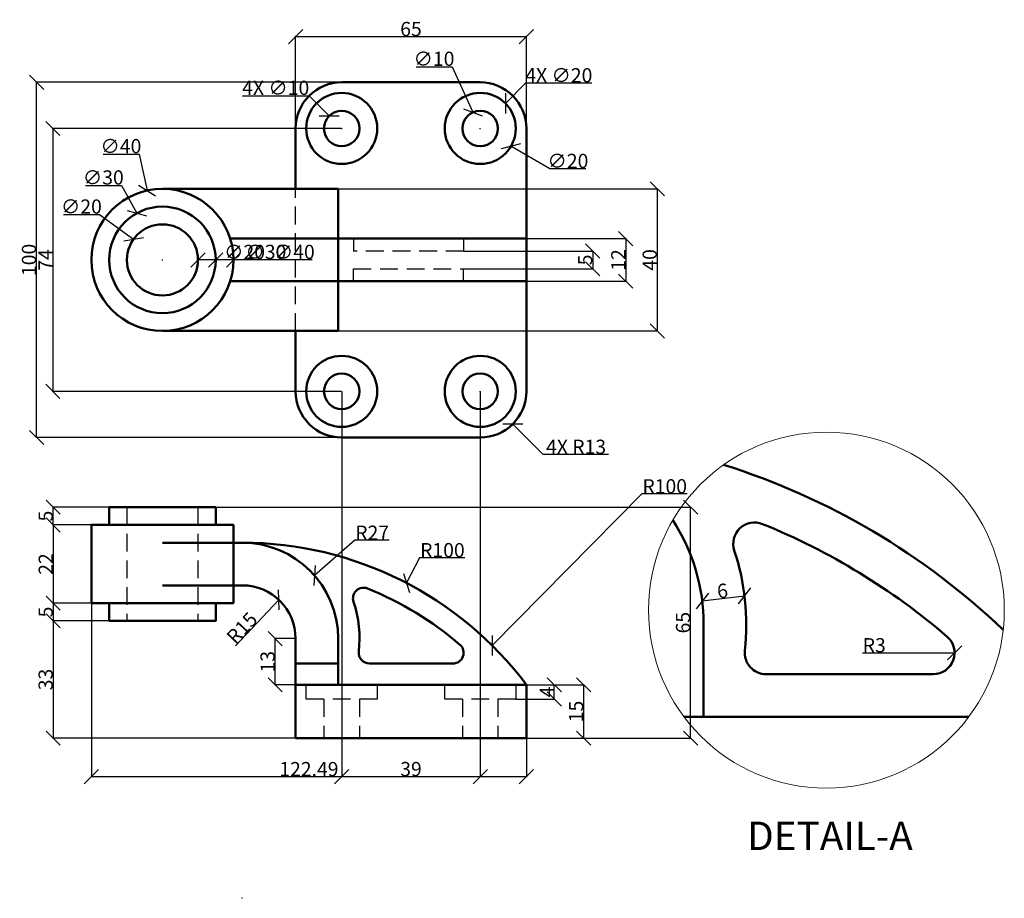
# Model space of a CAD drawing. Units: millimetres. Extents: x 103 to 380, y 45 to 292.
import ezdxf

# ---------------------------------------------------------------- set-up
doc = ezdxf.new("R2010")
doc.units = ezdxf.units.MM
doc.header["$MEASUREMENT"] = 0
doc.linetypes.add('HIDDEN', pattern=[0.375, 0.25, -0.125])
for name, color, linetype, lineweight in [('M-ANNO-DETL', 7, 'Continuous', 18), ('M-DIMS', 2, 'Continuous', 25), ('M-HIDN', 8, 'HIDDEN', 25), ('M-OUTL', 7, 'Continuous', 50), ('M-TEXT', 7, 'Continuous', 25)]:
    doc.layers.add(name, color=color, linetype=linetype, lineweight=lineweight)
doc.styles.get("Standard").update_dxf_attribs({"font": 'arial.ttf'})
doc.dimstyles.get("Standard").update_dxf_attribs({"dimtxt": 4, "dimasz": 4, "dimexe": 0.18, "dimexo": 0.0625, "dimgap": 0.09, "dimtad": 1, "dimtoh": 1, "dimdec": 0, "dimzin": 0, "dimdsep": 46, "dimtxsty": 'Standard', "dimblk": 'OBLIQUE', "dimcen": 0.09, "dimclre": 251, "dimadec": 0, "dimazin": 0, "dimtfac": 1, "dimtdec": 0, "dimtofl": 0, "dimtmove": 0, "dimatfit": 3, "dimfxl": 1, "dimtolj": 1, "dimtzin": 0, "dimarcsym": 0})

# ---------------------------------------------------------------- blocks, each defined once
blk = doc.blocks.new('_Oblique')
at = {"color": 0, "linetype": 'ByBlock', "lineweight": -2}
blk.add_line((-0.5, -0.5), (0.5, 0.5), dxfattribs=at)
blk = doc.blocks.new('*D2')
at = {"layer": 'Defpoints', "color": 0, "transparency": 16777216}
for p in [(295.18, 128.35), (307.09, 129.82), (307.09, 129.82)]:
    blk.add_point(p, dxfattribs=at)
at = {"layer": 'M-DIMS', "color": 0, "lineweight": -2, "transparency": 16777216}
for p, q in [((295.17, 128.41), (295.16, 128.53)), ((295.18, 128.35), (307.09, 129.82)), ((307.08, 129.88), (307.07, 130))]:
    blk.add_line(p, q, dxfattribs=at)
at = {"layer": 'M-DIMS', "color": 0, "lineweight": -2, "transparency": 16777216, "xscale": 4, "yscale": 4, "zscale": 4}
for p, rotation in [((295.18, 128.35), 187.0192128226031), ((307.09, 129.82), 7.019212822603112)]:
    blk.add_blockref('_Oblique', p, dxfattribs=dict(at, rotation=rotation))
at = {"layer": 'M-DIMS', "color": 0, "transparency": 16777216, "insert": (300.87, 131.2), "char_height": 4, "attachment_point": 5, "rotation": 7.0192}
blk.add_mtext('\\A1;6', dxfattribs=at)
blk = doc.blocks.new('*D3')
at = {"layer": 'Defpoints', "color": 0, "transparency": 16777216}
for p in [(360.24, 113.75), (366.24, 113.75)]:
    blk.add_point(p, dxfattribs=at)
at = {"layer": 'M-DIMS', "color": 0, "lineweight": -2, "transparency": 16777216}
blk.add_line((340.3, 113.75), (366.24, 113.75), dxfattribs=at)
at = {"layer": 'M-DIMS', "color": 0, "lineweight": -2, "transparency": 16777216, "xscale": 4, "yscale": 4, "zscale": 4, "rotation": 1.0687e-12}
blk.add_blockref('_Oblique', (366.24, 113.75), dxfattribs=at)
at = {"layer": 'M-DIMS', "color": 0, "transparency": 16777216, "insert": (343.61, 115.89), "char_height": 4, "attachment_point": 5}
blk.add_mtext('\\A1;R3', dxfattribs=at)
blk = doc.blocks.new('*D4')
at = {"layer": 'Defpoints', "color": 0, "transparency": 16777216}
for p in [(107.75, 274.35), (193.67, 274.35), (193.67, 174.35)]:
    blk.add_point(p, dxfattribs=at)
at = {"layer": 'M-DIMS', "color": 0, "lineweight": -2, "transparency": 16777216}
for p, q in [((193.61, 274.35), (107.57, 274.35)), ((107.75, 174.35), (107.75, 274.35)), ((193.61, 174.35), (107.57, 174.35))]:
    blk.add_line(p, q, dxfattribs=at)
at = {"layer": 'M-DIMS', "color": 0, "lineweight": -2, "transparency": 16777216, "xscale": 4, "yscale": 4, "zscale": 4}
for p, rotation in [((107.75, 274.35), 90), ((107.75, 174.35), 270)]:
    blk.add_blockref('_Oblique', p, dxfattribs=dict(at, rotation=rotation))
at = {"layer": 'M-DIMS', "color": 0, "transparency": 16777216, "insert": (105.61, 224.35), "char_height": 4, "attachment_point": 5, "rotation": 90}
blk.add_mtext('\\A1;100', dxfattribs=at)
blk = doc.blocks.new('*D5')
at = {"layer": 'Defpoints', "color": 0, "transparency": 16777216}
for p in [(228, 226.85), (228, 221.85), (264.33, 221.85)]:
    blk.add_point(p, dxfattribs=at)
at = {"layer": 'M-DIMS', "color": 0, "lineweight": -2, "transparency": 16777216}
for p, q in [((228.06, 226.85), (264.51, 226.85)), ((264.33, 226.85), (264.33, 221.85)), ((228.06, 221.85), (264.51, 221.85))]:
    blk.add_line(p, q, dxfattribs=at)
at = {"layer": 'M-DIMS', "color": 0, "lineweight": -2, "transparency": 16777216, "xscale": 4, "yscale": 4, "zscale": 4}
for p, rotation in [((264.33, 226.85), 90), ((264.33, 221.85), 270)]:
    blk.add_blockref('_Oblique', p, dxfattribs=dict(at, rotation=rotation))
at = {"layer": 'M-DIMS', "color": 0, "transparency": 16777216, "insert": (262.2, 224.35), "char_height": 4, "attachment_point": 5, "rotation": 90}
blk.add_mtext('\\A1;5', dxfattribs=at)
blk = doc.blocks.new('*D6')
at = {"layer": 'Defpoints', "color": 0, "transparency": 16777216}
for p in [(245.67, 230.35), (245.67, 218.35), (273.64, 218.35)]:
    blk.add_point(p, dxfattribs=at)
at = {"layer": 'M-DIMS', "color": 0, "lineweight": -2, "transparency": 16777216}
for p, q in [((245.73, 230.35), (273.82, 230.35)), ((273.64, 230.35), (273.64, 218.35)), ((245.73, 218.35), (273.82, 218.35))]:
    blk.add_line(p, q, dxfattribs=at)
at = {"layer": 'M-DIMS', "color": 0, "lineweight": -2, "transparency": 16777216, "xscale": 4, "yscale": 4, "zscale": 4}
for p, rotation in [((273.64, 230.35), 90), ((273.64, 218.35), 270)]:
    blk.add_blockref('_Oblique', p, dxfattribs=dict(at, rotation=rotation))
at = {"layer": 'M-DIMS', "color": 0, "transparency": 16777216, "insert": (271.54, 224.35), "char_height": 4, "attachment_point": 5, "rotation": 90}
blk.add_mtext('\\A1;12', dxfattribs=at)
blk = doc.blocks.new('*D7')
at = {"layer": 'Defpoints', "color": 0, "transparency": 16777216}
for p in [(192.67, 244.35), (192.67, 204.35), (282.53, 204.35)]:
    blk.add_point(p, dxfattribs=at)
at = {"layer": 'M-DIMS', "color": 0, "lineweight": -2, "transparency": 16777216}
for p, q in [((192.73, 244.35), (282.71, 244.35)), ((282.53, 244.35), (282.53, 204.35)), ((192.73, 204.35), (282.71, 204.35))]:
    blk.add_line(p, q, dxfattribs=at)
at = {"layer": 'M-DIMS', "color": 0, "lineweight": -2, "transparency": 16777216, "xscale": 4, "yscale": 4, "zscale": 4}
for p, rotation in [((282.53, 244.35), 90), ((282.53, 204.35), 270)]:
    blk.add_blockref('_Oblique', p, dxfattribs=dict(at, rotation=rotation))
at = {"layer": 'M-DIMS', "color": 0, "transparency": 16777216, "insert": (280.4, 224.35), "char_height": 4, "attachment_point": 5, "rotation": 90}
blk.add_mtext('\\A1;40', dxfattribs=at)
blk = doc.blocks.new('*D8')
at = {"layer": 'Defpoints', "color": 0, "transparency": 16777216}
for p in [(245.67, 287.2), (180.67, 261.35), (245.67, 261.35)]:
    blk.add_point(p, dxfattribs=at)
at = {"layer": 'M-DIMS', "color": 0, "lineweight": -2, "transparency": 16777216}
for p, q in [((180.67, 261.42), (180.67, 287.38)), ((180.67, 287.2), (245.67, 287.2)), ((245.67, 261.42), (245.67, 287.38))]:
    blk.add_line(p, q, dxfattribs=at)
at = {"layer": 'M-DIMS', "color": 0, "lineweight": -2, "transparency": 16777216, "xscale": 4, "yscale": 4, "zscale": 4, "rotation": 180}
blk.add_blockref('_Oblique', (180.67, 287.2), dxfattribs=at)
at = {"layer": 'M-DIMS', "color": 0, "lineweight": -2, "transparency": 16777216, "xscale": 4, "yscale": 4, "zscale": 4}
blk.add_blockref('_Oblique', (245.67, 287.2), dxfattribs=at)
at = {"layer": 'M-DIMS', "color": 0, "transparency": 16777216, "insert": (213.17, 289.34), "char_height": 4, "attachment_point": 5}
blk.add_mtext('\\A1;65', dxfattribs=at)
blk = doc.blocks.new('*D9')
at = {"layer": 'Defpoints', "color": 0, "transparency": 16777216}
for p in [(224.03, 266.38), (241.31, 256.32)]:
    blk.add_point(p, dxfattribs=at)
at = {"layer": 'M-DIMS', "color": 0, "lineweight": -2, "transparency": 16777216}
for p, q in [((232.58, 261.35), (232.76, 261.35)), ((232.67, 261.26), (232.67, 261.44)), ((252.24, 249.97), (241.31, 256.32)), ((262.4, 249.97), (252.24, 249.97))]:
    blk.add_line(p, q, dxfattribs=at)
at = {"layer": 'M-DIMS', "color": 0, "lineweight": -2, "transparency": 16777216, "xscale": 4, "yscale": 4, "zscale": 4, "rotation": 149.8067567273419}
blk.add_blockref('_Oblique', (241.31, 256.32), dxfattribs=at)
at = {"layer": 'M-DIMS', "color": 0, "transparency": 16777216, "insert": (257.36, 252.21), "char_height": 4, "attachment_point": 5}
blk.add_mtext('\\A1;∅20', dxfattribs=at)
blk = doc.blocks.new('*D10')
at = {"layer": 'Defpoints', "color": 0, "transparency": 16777216}
for p in [(230.6, 265.91), (234.74, 256.8)]:
    blk.add_point(p, dxfattribs=at)
at = {"layer": 'M-DIMS', "color": 0, "lineweight": -2, "transparency": 16777216}
for p, q in [((214.62, 278.72), (224.78, 278.72)), ((224.78, 278.72), (230.6, 265.91)), ((232.58, 261.35), (232.76, 261.35)), ((232.67, 261.26), (232.67, 261.44))]:
    blk.add_line(p, q, dxfattribs=at)
at = {"layer": 'M-DIMS', "color": 0, "lineweight": -2, "transparency": 16777216, "xscale": 4, "yscale": 4, "zscale": 4, "rotation": 294.4447376869272}
blk.add_blockref('_Oblique', (230.6, 265.91), dxfattribs=at)
at = {"layer": 'M-DIMS', "color": 0, "transparency": 16777216, "insert": (219.65, 280.96), "char_height": 4, "attachment_point": 5}
blk.add_mtext('\\A1;∅10', dxfattribs=at)
blk = doc.blocks.new('*D11')
at = {"layer": 'Defpoints', "color": 0, "transparency": 16777216}
for p in [(138.87, 243.88), (147.5, 204.82)]:
    blk.add_point(p, dxfattribs=at)
at = {"layer": 'M-DIMS', "color": 0, "lineweight": -2, "transparency": 16777216}
for p, q in [((126.45, 254.13), (136.61, 254.13)), ((136.61, 254.13), (138.87, 243.88)), ((143.09, 224.35), (143.27, 224.35)), ((143.18, 224.26), (143.18, 224.44))]:
    blk.add_line(p, q, dxfattribs=at)
at = {"layer": 'M-DIMS', "color": 0, "lineweight": -2, "transparency": 16777216, "xscale": 4, "yscale": 4, "zscale": 4, "rotation": 282.4485269081785}
blk.add_blockref('_Oblique', (138.87, 243.88), dxfattribs=at)
at = {"layer": 'M-DIMS', "color": 0, "transparency": 16777216, "insert": (131.49, 256.37), "char_height": 4, "attachment_point": 5}
blk.add_mtext('\\A1;∅40', dxfattribs=at)
blk = doc.blocks.new('*D12')
at = {"layer": 'Defpoints', "color": 0, "transparency": 16777216}
for p in [(135.96, 237.5), (150.41, 211.21)]:
    blk.add_point(p, dxfattribs=at)
at = {"layer": 'M-DIMS', "color": 0, "lineweight": -2, "transparency": 16777216}
for p, q in [((121.5, 245.32), (131.66, 245.32)), ((131.66, 245.32), (135.96, 237.5)), ((143.09, 224.35), (143.27, 224.35)), ((143.18, 224.26), (143.18, 224.44))]:
    blk.add_line(p, q, dxfattribs=at)
at = {"layer": 'M-DIMS', "color": 0, "lineweight": -2, "transparency": 16777216, "xscale": 4, "yscale": 4, "zscale": 4, "rotation": 298.8019066556523}
blk.add_blockref('_Oblique', (135.96, 237.5), dxfattribs=at)
at = {"layer": 'M-DIMS', "color": 0, "transparency": 16777216, "insert": (126.53, 247.56), "char_height": 4, "attachment_point": 5}
blk.add_mtext('\\A1;∅30', dxfattribs=at)
blk = doc.blocks.new('*D13')
at = {"layer": 'Defpoints', "color": 0, "transparency": 16777216}
for p in [(135.08, 230.21), (151.29, 218.5)]:
    blk.add_point(p, dxfattribs=at)
at = {"layer": 'M-DIMS', "color": 0, "lineweight": -2, "transparency": 16777216}
for p, q in [((115.33, 237.13), (125.49, 237.13)), ((125.49, 237.13), (135.08, 230.21)), ((143.09, 224.35), (143.27, 224.35)), ((143.18, 224.26), (143.18, 224.44))]:
    blk.add_line(p, q, dxfattribs=at)
at = {"layer": 'M-DIMS', "color": 0, "lineweight": -2, "transparency": 16777216, "xscale": 4, "yscale": 4, "zscale": 4, "rotation": 324.1807980481107}
blk.add_blockref('_Oblique', (135.08, 230.21), dxfattribs=at)
at = {"layer": 'M-DIMS', "color": 0, "transparency": 16777216, "insert": (120.36, 239.37), "char_height": 4, "attachment_point": 5}
blk.add_mtext('\\A1;∅20', dxfattribs=at)
blk = doc.blocks.new('*D14')
at = {"layer": 'Defpoints', "color": 0, "transparency": 16777216}
for p in [(112.43, 154.75), (128.18, 154.75), (123.18, 149.75)]:
    blk.add_point(p, dxfattribs=at)
at = {"layer": 'M-DIMS', "color": 0, "lineweight": -2, "transparency": 16777216}
for p, q in [((128.12, 154.75), (112.25, 154.75)), ((112.43, 149.75), (112.43, 154.75)), ((123.12, 149.75), (112.25, 149.75))]:
    blk.add_line(p, q, dxfattribs=at)
at = {"layer": 'M-DIMS', "color": 0, "lineweight": -2, "transparency": 16777216, "xscale": 4, "yscale": 4, "zscale": 4}
for p, rotation in [((112.43, 154.75), 90), ((112.43, 149.75), 270)]:
    blk.add_blockref('_Oblique', p, dxfattribs=dict(at, rotation=rotation))
at = {"layer": 'M-DIMS', "color": 0, "transparency": 16777216, "insert": (110.3, 152.25), "char_height": 4, "attachment_point": 5, "rotation": 90}
blk.add_mtext('\\A1;5', dxfattribs=at)
blk = doc.blocks.new('*D15')
at = {"layer": 'Defpoints', "color": 0, "transparency": 16777216}
for p in [(123.18, 149.75), (112.43, 127.75), (123.18, 127.75)]:
    blk.add_point(p, dxfattribs=at)
at = {"layer": 'M-DIMS', "color": 0, "lineweight": -2, "transparency": 16777216}
for p, q in [((123.12, 149.75), (112.25, 149.75)), ((112.43, 149.75), (112.43, 127.75)), ((123.12, 127.75), (112.25, 127.75))]:
    blk.add_line(p, q, dxfattribs=at)
at = {"layer": 'M-DIMS', "color": 0, "lineweight": -2, "transparency": 16777216, "xscale": 4, "yscale": 4, "zscale": 4}
for p, rotation in [((112.43, 149.75), 90), ((112.43, 127.75), 270)]:
    blk.add_blockref('_Oblique', p, dxfattribs=dict(at, rotation=rotation))
at = {"layer": 'M-DIMS', "color": 0, "transparency": 16777216, "insert": (110.33, 138.75), "char_height": 4, "attachment_point": 5, "rotation": 90}
blk.add_mtext('\\A1;22', dxfattribs=at)
blk = doc.blocks.new('*D16')
at = {"layer": 'Defpoints', "color": 0, "transparency": 16777216}
for p in [(123.18, 127.75), (112.43, 122.75), (128.18, 122.75)]:
    blk.add_point(p, dxfattribs=at)
at = {"layer": 'M-DIMS', "color": 0, "lineweight": -2, "transparency": 16777216}
for p, q in [((123.12, 127.75), (112.25, 127.75)), ((112.43, 127.75), (112.43, 122.75)), ((128.12, 122.75), (112.25, 122.75))]:
    blk.add_line(p, q, dxfattribs=at)
at = {"layer": 'M-DIMS', "color": 0, "lineweight": -2, "transparency": 16777216, "xscale": 4, "yscale": 4, "zscale": 4}
for p, rotation in [((112.43, 127.75), 90), ((112.43, 122.75), 270)]:
    blk.add_blockref('_Oblique', p, dxfattribs=dict(at, rotation=rotation))
at = {"layer": 'M-DIMS', "color": 0, "transparency": 16777216, "insert": (110.3, 125.25), "char_height": 4, "attachment_point": 5, "rotation": 90}
blk.add_mtext('\\A1;5', dxfattribs=at)
blk = doc.blocks.new('*D17')
at = {"layer": 'Defpoints', "color": 0, "transparency": 16777216}
for p in [(128.18, 122.75), (112.43, 89.75), (180.67, 89.75)]:
    blk.add_point(p, dxfattribs=at)
at = {"layer": 'M-DIMS', "color": 0, "lineweight": -2, "transparency": 16777216}
for p, q in [((128.12, 122.75), (112.25, 122.75)), ((112.43, 122.75), (112.43, 89.75)), ((180.61, 89.75), (112.25, 89.75))]:
    blk.add_line(p, q, dxfattribs=at)
at = {"layer": 'M-DIMS', "color": 0, "lineweight": -2, "transparency": 16777216, "xscale": 4, "yscale": 4, "zscale": 4}
for p, rotation in [((112.43, 122.75), 90), ((112.43, 89.75), 270)]:
    blk.add_blockref('_Oblique', p, dxfattribs=dict(at, rotation=rotation))
at = {"layer": 'M-DIMS', "color": 0, "transparency": 16777216, "insert": (110.29, 106.25), "char_height": 4, "attachment_point": 5, "rotation": 90}
blk.add_mtext('\\A1;33', dxfattribs=at)
blk = doc.blocks.new('*D18')
at = {"layer": 'Defpoints', "color": 0, "transparency": 16777216}
for p in [(174.93, 117.75), (180.67, 117.75), (180.67, 104.75)]:
    blk.add_point(p, dxfattribs=at)
at = {"layer": 'M-DIMS', "color": 0, "lineweight": -2, "transparency": 16777216}
for p, q in [((180.61, 117.75), (174.75, 117.75)), ((174.93, 104.75), (174.93, 117.75)), ((180.61, 104.75), (174.75, 104.75))]:
    blk.add_line(p, q, dxfattribs=at)
at = {"layer": 'M-DIMS', "color": 0, "lineweight": -2, "transparency": 16777216, "xscale": 4, "yscale": 4, "zscale": 4}
for p, rotation in [((174.93, 117.75), 90), ((174.93, 104.75), 270)]:
    blk.add_blockref('_Oblique', p, dxfattribs=dict(at, rotation=rotation))
at = {"layer": 'M-DIMS', "color": 0, "transparency": 16777216, "insert": (172.8, 111.25), "char_height": 4, "attachment_point": 5, "rotation": 90}
blk.add_mtext('\\A1;13', dxfattribs=at)
blk = doc.blocks.new('*D19')
at = {"layer": 'Defpoints', "color": 0, "transparency": 16777216}
for p in [(245.67, 104.75), (253.53, 104.75), (242.67, 100.75)]:
    blk.add_point(p, dxfattribs=at)
at = {"layer": 'M-DIMS', "color": 0, "lineweight": -2, "transparency": 16777216}
for p, q in [((245.73, 104.75), (253.71, 104.75)), ((253.53, 100.75), (253.53, 104.75)), ((242.73, 100.75), (253.71, 100.75))]:
    blk.add_line(p, q, dxfattribs=at)
at = {"layer": 'M-DIMS', "color": 0, "lineweight": -2, "transparency": 16777216, "xscale": 4, "yscale": 4, "zscale": 4}
for p, rotation in [((253.53, 104.75), 90), ((253.53, 100.75), 270)]:
    blk.add_blockref('_Oblique', p, dxfattribs=dict(at, rotation=rotation))
at = {"layer": 'M-DIMS', "color": 0, "transparency": 16777216, "insert": (251.44, 102.75), "char_height": 4, "attachment_point": 5, "rotation": 90}
blk.add_mtext('\\A1;4', dxfattribs=at)
blk = doc.blocks.new('*D20')
at = {"layer": 'Defpoints', "color": 0, "transparency": 16777216}
for p in [(245.67, 104.75), (261.8, 104.75), (245.67, 89.75)]:
    blk.add_point(p, dxfattribs=at)
at = {"layer": 'M-DIMS', "color": 0, "lineweight": -2, "transparency": 16777216}
for p, q in [((245.73, 104.75), (261.98, 104.75)), ((261.8, 89.75), (261.8, 104.75)), ((245.73, 89.75), (261.98, 89.75))]:
    blk.add_line(p, q, dxfattribs=at)
at = {"layer": 'M-DIMS', "color": 0, "lineweight": -2, "transparency": 16777216, "xscale": 4, "yscale": 4, "zscale": 4}
for p, rotation in [((261.8, 104.75), 90), ((261.8, 89.75), 270)]:
    blk.add_blockref('_Oblique', p, dxfattribs=dict(at, rotation=rotation))
at = {"layer": 'M-DIMS', "color": 0, "transparency": 16777216, "insert": (259.67, 97.25), "char_height": 4, "attachment_point": 5, "rotation": 90}
blk.add_mtext('\\A1;15', dxfattribs=at)
blk = doc.blocks.new('*D21')
at = {"layer": 'Defpoints', "color": 0, "transparency": 16777216}
for p in [(186, 135.52), (165.67, 117.75)]:
    blk.add_point(p, dxfattribs=at)
at = {"layer": 'M-DIMS', "color": 0, "lineweight": -2, "transparency": 16777216}
for p, q in [((197.37, 145.47), (186, 135.52)), ((207.02, 145.47), (197.37, 145.47)), ((165.58, 117.75), (165.76, 117.75)), ((165.67, 117.66), (165.67, 117.84))]:
    blk.add_line(p, q, dxfattribs=at)
at = {"layer": 'M-DIMS', "color": 0, "lineweight": -2, "transparency": 16777216, "xscale": 4, "yscale": 4, "zscale": 4, "rotation": 221.1569914641529}
blk.add_blockref('_Oblique', (186, 135.52), dxfattribs=at)
at = {"layer": 'M-DIMS', "color": 0, "transparency": 16777216, "insert": (202.24, 147.56), "char_height": 4, "attachment_point": 5}
blk.add_mtext('\\A1;R27', dxfattribs=at)
blk = doc.blocks.new('*D22')
at = {"layer": 'Defpoints', "color": 0, "transparency": 16777216}
for p in [(175.95, 128.68), (165.67, 117.75)]:
    blk.add_point(p, dxfattribs=at)
at = {"layer": 'M-DIMS', "color": 0, "lineweight": -2, "transparency": 16777216}
blk.add_line((163.77, 115.74), (175.95, 128.68), dxfattribs=at)
at = {"layer": 'M-DIMS', "color": 0, "lineweight": -2, "transparency": 16777216, "xscale": 4, "yscale": 4, "zscale": 4, "rotation": 46.76402334800748}
blk.add_blockref('_Oblique', (175.95, 128.68), dxfattribs=at)
at = {"layer": 'M-DIMS', "color": 0, "transparency": 16777216, "insert": (165.57, 120.75), "char_height": 4, "attachment_point": 5, "rotation": 46.764}
blk.add_mtext('\\A1;R15', dxfattribs=at)
blk = doc.blocks.new('*D23')
at = {"layer": 'Defpoints', "color": 0, "transparency": 16777216}
for p in [(211.9, 133.42), (165.67, 44.75)]:
    blk.add_point(p, dxfattribs=at)
at = {"layer": 'M-DIMS', "color": 0, "lineweight": -2, "transparency": 16777216}
for p, q in [((215.6, 140.52), (211.9, 133.42)), ((228.34, 140.52), (215.6, 140.52)), ((165.58, 44.75), (165.76, 44.75)), ((165.67, 44.66), (165.67, 44.84))]:
    blk.add_line(p, q, dxfattribs=at)
at = {"layer": 'M-DIMS', "color": 0, "lineweight": -2, "transparency": 16777216, "xscale": 4, "yscale": 4, "zscale": 4, "rotation": 242.4630051083834}
blk.add_blockref('_Oblique', (211.9, 133.42), dxfattribs=at)
at = {"layer": 'M-DIMS', "color": 0, "transparency": 16777216, "insert": (222.02, 142.65), "char_height": 4, "attachment_point": 5}
blk.add_mtext('\\A1;R100', dxfattribs=at)
blk = doc.blocks.new('BASE-HOLE-D10-CBORE-D20-PLAN')
for radius in [10, 5]:
    blk.add_circle((0, 0), radius)
blk = doc.blocks.new('BASE-HOLE-D10-CBORE-D20-ELEV')
at = {"ltscale": 20}
for p, q in [((-10, -4), (-10, 0)), ((10, 0), (10, -4)), ((10, -4), (-10, -4)), ((-5, -4), (-5, -15)), ((5, -4), (5, -15))]:
    blk.add_line(p, q, dxfattribs=at)
blk = doc.blocks.new('WEB-RECESS-PLAN')
at = {"ltscale": 20}
for p, q in [((0, 3.5), (31.01, 3.5)), ((0, 0), (0, 3.5)), ((31.01, 0), (31.01, 3.5))]:
    blk.add_line(p, q, dxfattribs=at)
blk = doc.blocks.new('*D27')
at = {"layer": 'Defpoints', "color": 0, "transparency": 16777216}
for p in [(123.18, 127.75), (245.67, 89.75), (245.67, 78.9)]:
    blk.add_point(p, dxfattribs=at)
at = {"layer": 'M-DIMS', "color": 251, "lineweight": -2, "transparency": 16777216}
for p, q in [((123.18, 127.69), (123.18, 78.72)), ((245.67, 89.69), (245.67, 78.72))]:
    blk.add_line(p, q, dxfattribs=at)
at = {"layer": 'M-DIMS', "color": 0, "lineweight": -2, "transparency": 16777216}
blk.add_line((123.18, 78.9), (245.67, 78.9), dxfattribs=at)
at = {"layer": 'M-DIMS', "color": 0, "lineweight": -2, "transparency": 16777216, "xscale": 4, "yscale": 4, "zscale": 4, "rotation": 180}
blk.add_blockref('_Oblique', (123.18, 78.9), dxfattribs=at)
at = {"layer": 'M-DIMS', "color": 0, "lineweight": -2, "transparency": 16777216, "xscale": 4, "yscale": 4, "zscale": 4}
blk.add_blockref('_Oblique', (245.67, 78.9), dxfattribs=at)
at = {"layer": 'M-DIMS', "color": 0, "transparency": 16777216, "insert": (184.43, 81.03), "char_height": 4, "attachment_point": 5}
blk.add_mtext('\\A1;122.49', dxfattribs=at)
blk = doc.blocks.new('*D28')
at = {"layer": 'Defpoints', "color": 0, "transparency": 16777216}
for p in [(158.18, 154.75), (291.91, 154.75), (245.67, 89.75)]:
    blk.add_point(p, dxfattribs=at)
at = {"layer": 'M-DIMS', "color": 251, "lineweight": -2, "transparency": 16777216}
for p, q in [((158.25, 154.75), (292.09, 154.75)), ((245.73, 89.75), (292.09, 89.75))]:
    blk.add_line(p, q, dxfattribs=at)
at = {"layer": 'M-DIMS', "color": 0, "lineweight": -2, "transparency": 16777216}
blk.add_line((291.91, 89.75), (291.91, 154.75), dxfattribs=at)
at = {"layer": 'M-DIMS', "color": 0, "lineweight": -2, "transparency": 16777216, "xscale": 4, "yscale": 4, "zscale": 4}
for p, rotation in [((291.91, 154.75), 90), ((291.91, 89.75), 270)]:
    blk.add_blockref('_Oblique', p, dxfattribs=dict(at, rotation=rotation))
at = {"layer": 'M-DIMS', "color": 0, "transparency": 16777216, "insert": (289.78, 122.25), "char_height": 4, "attachment_point": 5, "rotation": 90}
blk.add_mtext('\\A1;65', dxfattribs=at)
blk = doc.blocks.new('*D29')
at = {"layer": 'Defpoints', "color": 0, "transparency": 16777216}
for p in [(193.67, 187.35), (232.67, 187.35), (232.67, 78.9)]:
    blk.add_point(p, dxfattribs=at)
at = {"layer": 'M-DIMS', "color": 251, "lineweight": -2, "transparency": 16777216}
for p, q in [((193.67, 187.29), (193.67, 78.72)), ((232.67, 187.29), (232.67, 78.72))]:
    blk.add_line(p, q, dxfattribs=at)
at = {"layer": 'M-DIMS', "color": 0, "lineweight": -2, "transparency": 16777216}
blk.add_line((193.67, 78.9), (232.67, 78.9), dxfattribs=at)
at = {"layer": 'M-DIMS', "color": 0, "lineweight": -2, "transparency": 16777216, "xscale": 4, "yscale": 4, "zscale": 4, "rotation": 180}
blk.add_blockref('_Oblique', (193.67, 78.9), dxfattribs=at)
at = {"layer": 'M-DIMS', "color": 0, "lineweight": -2, "transparency": 16777216, "xscale": 4, "yscale": 4, "zscale": 4}
blk.add_blockref('_Oblique', (232.67, 78.9), dxfattribs=at)
at = {"layer": 'M-DIMS', "color": 0, "transparency": 16777216, "insert": (213.17, 81.04), "char_height": 4, "attachment_point": 5}
blk.add_mtext('\\A1;39', dxfattribs=at)
blk = doc.blocks.new('*D30')
at = {"layer": 'Defpoints', "color": 0, "transparency": 16777216}
for p in [(193.670085, 261.353741), (112.334331, 187.353741), (193.670085, 187.353741)]:
    blk.add_point(p, dxfattribs=at)
at = {"layer": 'M-DIMS', "color": 251, "lineweight": -2, "transparency": 16777216}
for p, q in [((193.607585, 261.353741), (112.154331, 261.353741)), ((193.607585, 187.353741), (112.154331, 187.353741))]:
    blk.add_line(p, q, dxfattribs=at)
at = {"layer": 'M-DIMS', "color": 0, "lineweight": -2, "transparency": 16777216}
blk.add_line((112.334331, 261.353741), (112.334331, 187.353741), dxfattribs=at)
at = {"layer": 'M-DIMS', "color": 0, "lineweight": -2, "transparency": 16777216, "xscale": 4, "yscale": 4, "zscale": 4}
for p, rotation in [((112.334331, 261.353741), 90), ((112.334331, 187.353741), 270)]:
    blk.add_blockref('_Oblique', p, dxfattribs=dict(at, rotation=rotation))
at = {"layer": 'M-DIMS', "color": 0, "transparency": 16777216, "insert": (110.244331, 224.353741), "char_height": 4, "attachment_point": 5, "rotation": 90}
blk.add_mtext('\\A1;74', dxfattribs=at)
blk = doc.blocks.new('*D31')
at = {"layer": 'Defpoints', "color": 0, "transparency": 16777216}
for p in [(232.67, 187.35), (241.86, 178.16)]:
    blk.add_point(p, dxfattribs=at)
at = {"layer": 'M-DIMS', "color": 251, "lineweight": -2, "transparency": 16777216}
for p, q in [((232.58, 187.35), (232.76, 187.35)), ((232.67, 187.26), (232.67, 187.44))]:
    blk.add_line(p, q, dxfattribs=at)
at = {"layer": 'M-DIMS', "color": 0, "lineweight": -2, "transparency": 16777216}
for p, q in [((250.41, 169.61), (241.86, 178.16)), ((268.81, 169.61), (250.41, 169.61))]:
    blk.add_line(p, q, dxfattribs=at)
at = {"layer": 'M-DIMS', "color": 0, "lineweight": -2, "transparency": 16777216, "xscale": 4, "yscale": 4, "zscale": 4, "rotation": 134.9974257878445}
blk.add_blockref('_Oblique', (241.86, 178.16), dxfattribs=at)
at = {"layer": 'M-DIMS', "color": 0, "transparency": 16777216, "insert": (259.66, 171.75), "char_height": 4, "attachment_point": 5}
blk.add_mtext('\\A1;4X R13', dxfattribs=at)
blk = doc.blocks.new('*D32')
at = {"layer": 'Defpoints', "color": 0, "transparency": 16777216}
for p in [(239.74, 268.42), (225.6, 254.28)]:
    blk.add_point(p, dxfattribs=at)
at = {"layer": 'M-DIMS', "color": 0, "lineweight": -2, "transparency": 16777216}
for p, q in [((245.4, 274.08), (239.74, 268.42)), ((264.1, 274.08), (245.4, 274.08))]:
    blk.add_line(p, q, dxfattribs=at)
at = {"layer": 'M-DIMS', "color": 251, "lineweight": -2, "transparency": 16777216}
for p, q in [((232.58, 261.35), (232.76, 261.35)), ((232.67, 261.26), (232.67, 261.44))]:
    blk.add_line(p, q, dxfattribs=at)
at = {"layer": 'M-DIMS', "color": 0, "lineweight": -2, "transparency": 16777216, "xscale": 4, "yscale": 4, "zscale": 4, "rotation": 224.98518394422}
blk.add_blockref('_Oblique', (239.74, 268.42), dxfattribs=at)
at = {"layer": 'M-DIMS', "color": 0, "transparency": 16777216, "insert": (254.8, 276.32), "char_height": 4, "attachment_point": 5}
blk.add_mtext('\\A1;4X ∅20', dxfattribs=at)
blk = doc.blocks.new('*D33')
at = {"layer": 'Defpoints', "color": 0, "transparency": 16777216}
for p in [(190.13, 264.89), (197.21, 257.82)]:
    blk.add_point(p, dxfattribs=at)
at = {"layer": 'M-DIMS', "color": 0, "lineweight": -2, "transparency": 16777216}
for p, q in [((165.77, 270.54), (184.47, 270.54)), ((184.47, 270.54), (190.13, 264.89))]:
    blk.add_line(p, q, dxfattribs=at)
at = {"layer": 'M-DIMS', "color": 251, "lineweight": -2, "transparency": 16777216}
for p, q in [((193.58, 261.35), (193.76, 261.35)), ((193.67, 261.26), (193.67, 261.44))]:
    blk.add_line(p, q, dxfattribs=at)
at = {"layer": 'M-DIMS', "color": 0, "lineweight": -2, "transparency": 16777216, "xscale": 4, "yscale": 4, "zscale": 4, "rotation": 315.0309771840286}
blk.add_blockref('_Oblique', (190.13, 264.89), dxfattribs=at)
at = {"layer": 'M-DIMS', "color": 0, "transparency": 16777216, "insert": (175.08, 272.79), "char_height": 4, "attachment_point": 5}
blk.add_mtext('\\A1;4X ∅10', dxfattribs=at)
blk = doc.blocks.new('*D34')
at = {"layer": 'Defpoints', "color": 0, "transparency": 16777216}
for p in [(123.18, 224.35), (163.18, 224.35)]:
    blk.add_point(p, dxfattribs=at)
at = {"layer": 'M-DIMS', "color": 251, "lineweight": -2, "transparency": 16777216}
for p, q in [((143.09, 224.35), (143.27, 224.35)), ((143.18, 224.26), (143.18, 224.44))]:
    blk.add_line(p, q, dxfattribs=at)
at = {"layer": 'M-DIMS', "color": 0, "lineweight": -2, "transparency": 16777216}
for p, q in [((175.18, 224.35), (163.18, 224.35)), ((185.34, 224.35), (175.18, 224.35))]:
    blk.add_line(p, q, dxfattribs=at)
at = {"layer": 'M-DIMS', "color": 0, "lineweight": -2, "transparency": 16777216, "xscale": 4, "yscale": 4, "zscale": 4, "rotation": 180.0007419803447}
blk.add_blockref('_Oblique', (163.18, 224.35), dxfattribs=at)
at = {"layer": 'M-DIMS', "color": 0, "transparency": 16777216, "insert": (180.31, 226.6), "char_height": 4, "attachment_point": 5}
blk.add_mtext('\\A1;∅40', dxfattribs=at)
blk = doc.blocks.new('*D35')
at = {"layer": 'Defpoints', "color": 0, "transparency": 16777216}
for p in [(128.18, 224.35), (158.18, 224.35)]:
    blk.add_point(p, dxfattribs=at)
at = {"layer": 'M-DIMS', "color": 251, "lineweight": -2, "transparency": 16777216}
for p, q in [((143.09, 224.35), (143.27, 224.35)), ((143.18, 224.26), (143.18, 224.44))]:
    blk.add_line(p, q, dxfattribs=at)
at = {"layer": 'M-DIMS', "color": 0, "lineweight": -2, "transparency": 16777216}
for p, q in [((167.18, 224.35), (158.18, 224.35)), ((177.34, 224.35), (167.18, 224.35))]:
    blk.add_line(p, q, dxfattribs=at)
at = {"layer": 'M-DIMS', "color": 0, "lineweight": -2, "transparency": 16777216, "xscale": 4, "yscale": 4, "zscale": 4, "rotation": 180.0009893071261}
blk.add_blockref('_Oblique', (158.18, 224.35), dxfattribs=at)
at = {"layer": 'M-DIMS', "color": 0, "transparency": 16777216, "insert": (172.31, 226.6), "char_height": 4, "attachment_point": 5}
blk.add_mtext('\\A1;∅30', dxfattribs=at)
blk = doc.blocks.new('*D36')
at = {"layer": 'Defpoints', "color": 0, "transparency": 16777216}
for p in [(133.18, 224.35), (153.18, 224.35)]:
    blk.add_point(p, dxfattribs=at)
at = {"layer": 'M-DIMS', "color": 251, "lineweight": -2, "transparency": 16777216}
for p, q in [((143.09, 224.35), (143.27, 224.35)), ((143.18, 224.26), (143.18, 224.44))]:
    blk.add_line(p, q, dxfattribs=at)
at = {"layer": 'M-DIMS', "color": 0, "lineweight": -2, "transparency": 16777216}
for p, q in [((161.18, 224.35), (153.18, 224.35)), ((171.34, 224.35), (161.18, 224.35))]:
    blk.add_line(p, q, dxfattribs=at)
at = {"layer": 'M-DIMS', "color": 0, "lineweight": -2, "transparency": 16777216, "xscale": 4, "yscale": 4, "zscale": 4, "rotation": 180.001483960689}
blk.add_blockref('_Oblique', (153.18, 224.35), dxfattribs=at)
at = {"layer": 'M-DIMS', "color": 0, "transparency": 16777216, "insert": (166.31, 226.6), "char_height": 4, "attachment_point": 5}
blk.add_mtext('\\A1;∅20', dxfattribs=at)
blk = doc.blocks.new('*D37')
at = {"layer": 'Defpoints', "color": 0, "transparency": 16777216}
for p in [(236, 115.84), (165.67, 44.75)]:
    blk.add_point(p, dxfattribs=at)
at = {"layer": 'M-DIMS', "color": 0, "lineweight": -2, "transparency": 16777216}
for p, q in [((278.2, 158.49), (236, 115.84)), ((290.94, 158.49), (278.2, 158.49))]:
    blk.add_line(p, q, dxfattribs=at)
at = {"layer": 'M-DIMS', "color": 251, "lineweight": -2, "transparency": 16777216}
for p, q in [((165.58, 44.75), (165.76, 44.75)), ((165.67, 44.66), (165.67, 44.84))]:
    blk.add_line(p, q, dxfattribs=at)
at = {"layer": 'M-DIMS', "color": 0, "lineweight": -2, "transparency": 16777216, "xscale": 4, "yscale": 4, "zscale": 4, "rotation": 225.3069786326352}
blk.add_blockref('_Oblique', (236, 115.84), dxfattribs=at)
at = {"layer": 'M-DIMS', "color": 0, "transparency": 16777216, "insert": (284.62, 160.63), "char_height": 4, "attachment_point": 5}
blk.add_mtext('\\A1;R100', dxfattribs=at)

msp = doc.modelspace()

# ---------------------------------------------------------------- linework, layer by layer
at = {"layer": 'M-ANNO-DETL'}
msp.add_circle((330.142, 125.775), 50.1, dxfattribs=at)
at = {"layer": 'M-HIDN', "ltscale": 20}
for p, q in [((133.184, 154.752), (133.184, 122.752)), ((153.184, 154.752), (153.184, 122.752))]:
    msp.add_line(p, q, dxfattribs=at)
msp.add_lwpolyline([(180.67, 204.354), (180.67, 244.354)], dxfattribs=at)
at = {"layer": 'M-OUTL'}
for p, q in [((192.67, 244.354), (143.184, 244.354)), ((192.67, 244.354), (192.67, 204.354)), ((245.67, 230.354), (162.263, 230.354)), ((245.67, 218.354), (162.263, 218.354)), ((192.67, 204.354), (143.184, 204.354)), ((143.184, 144.752), (165.67, 144.752)), ((143.184, 132.752), (165.67, 132.752)), ((295.582, 95.752), (295.582, 121.752)), ((180.67, 104.752), (180.67, 117.752)), ((192.67, 104.752), (192.67, 117.752)), ((192.67, 110.752), (180.67, 110.752)), ((225, 110.752), (201.447, 110.752)), ((360.241, 107.752), (313.136, 107.752)), ((245.67, 104.752), (180.67, 104.752)), ((180.67, 89.752), (180.67, 104.752)), ((245.67, 89.752), (245.67, 104.752)), ((370.249, 95.752), (290.034, 95.752)), ((180.67, 89.752), (245.67, 89.752))]:
    msp.add_line(p, q, dxfattribs=at)
for points in [[(193.67, 274.354), (232.67, 274.354, -0.4142136), (245.67, 261.354), (245.67, 187.354, -0.4142136), (232.67, 174.354), (193.67, 174.354, -0.4142136), (180.67, 187.354), (180.67, 204.354)], [(180.67, 244.354), (180.67, 261.354, -0.4142136), (193.67, 274.354)]]:
    msp.add_lwpolyline(points, format="xyb", dxfattribs=at)
for points in [[(128.184, 149.752), (158.184, 149.752), (158.184, 154.752), (128.184, 154.752)], [(123.184, 149.752), (163.184, 149.752), (163.184, 127.752), (123.184, 127.752)], [(128.184, 127.752), (158.184, 127.752), (158.184, 122.752), (128.184, 122.752)]]:
    msp.add_lwpolyline(points, close=True, dxfattribs=at)
for centre, radius in [((143.184, 224.354), 20), ((143.184, 224.354), 15), ((143.184, 224.354), 10), ((193.67, 187.354), 10)]:
    msp.add_circle(centre, radius, dxfattribs=at)
for centre, radius, start, end in [((241.582, -24.248), 200, 46.23257, 72.66016), ((241.582, 121.752), 54, 0, 32.91812), ((309.915, 144.437), 6, 67.94751, 198.36495), ((241.582, -24.248), 188, 49.30944, 67.94751), ((165.67, 117.752), 27, 0, 90), ((165.67, 44.752), 100, 36.8699, 90), ((241.582, 121.752), 66, 353.62063, 18.36495), ((165.67, 117.752), 15, 0, 90), ((199.837, 129.095), 3, 67.94751, 198.36495), ((165.67, 44.752), 94, 49.30944, 67.94751), ((165.67, 117.752), 33, 353.62063, 18.36495), ((360.241, 113.752), 6, 270, 49.30944), ((201.447, 113.752), 3, 173.62063, 270), ((225, 113.752), 3, 270, 49.30944), ((313.136, 113.752), 6, 173.62063, 270)]:
    msp.add_arc(centre, radius, start, end, dxfattribs=at)

# ---------------------------------------------------------------- block references
at = {"layer": 'M-HIDN', "rotation": 180}
msp.add_blockref('WEB-RECESS-PLAN', (228, 230.354), dxfattribs=at)
at = {"layer": 'M-HIDN'}
for name, p in [('WEB-RECESS-PLAN', (196.987, 218.354)), ('BASE-HOLE-D10-CBORE-D20-ELEV', (193.67, 104.752)), ('BASE-HOLE-D10-CBORE-D20-ELEV', (232.67, 104.752))]:
    msp.add_blockref(name, p, dxfattribs=at)
at = {"layer": 'M-OUTL'}
for p in [(193.67, 261.354), (232.67, 261.354), (193.67, 187.354), (232.67, 187.354)]:
    msp.add_blockref('BASE-HOLE-D10-CBORE-D20-PLAN', p, dxfattribs=at)

# ---------------------------------------------------------------- texts
at = {"layer": 'M-TEXT', "insert": (307.819, 66.243), "char_height": 8, "attachment_point": 1}
msp.add_mtext_dynamic_manual_height_columns('DETAIL-A', width=73.57006, gutter_width=1, heights=[0], dxfattribs=at)

# ---------------------------------------------------------------- dimensions: what is measured, and where the dimension line sits
at = {"layer": 'M-DIMS'}
for base, p1, p2, override, picture, middle in [((245.67, 287.204), (180.67, 261.354), (245.67, 261.354), {"dimclrd": 0, "dimclre": 0, "dimclrt": 0}, '*D8', (213.17, 289.336)), ((232.67, 78.902), (193.67, 187.354), (232.67, 187.354), {"dimdec": 0, "dimlfac": 1, "dimrnd": 0, "dimzin": 0, "dimdsep": 46, "dimlunit": 2}, '*D29', (213.17, 81.036)), ((245.67, 78.902), (123.184, 127.752), (245.67, 89.752), {"dimdec": 2, "dimlfac": 1, "dimrnd": 0, "dimzin": 0, "dimdsep": 46, "dimlunit": 2}, '*D27', (184.427, 81.035))]:
    dim = msp.add_linear_dim(base=base, p1=p1, p2=p2, dimstyle='Standard', override=override, dxfattribs=at)
    dim.commit()
    dim.dimension.update_dxf_attribs({"geometry": picture, "text_midpoint": middle})
for p1, p2, override, picture, middle in [((234.739, 256.802), (230.601, 265.906), {"dimclrd": 0, "dimclre": 0, "dimclrt": 0}, '*D10', (219.653, 278.717)), ((224.027, 266.383), (241.313, 256.325), {"dimclrd": 0, "dimclre": 0, "dimclrt": 0}, '*D9', (257.361, 249.969)), ((147.496, 204.824), (138.873, 243.884), {"dimclrd": 0, "dimclre": 0, "dimclrt": 0}, '*D11', (131.488, 254.126)), ((150.411, 211.209), (135.958, 237.498), {"dimclrd": 0, "dimclre": 0, "dimclrt": 0}, '*D12', (126.534, 245.319)), ((151.293, 218.501), (135.076, 230.206), {"dimclrd": 0, "dimclre": 0, "dimclrt": 0}, '*D13', (120.362, 237.127)), ((123.184, 224.353), (163.184, 224.354), {"dimdec": 0, "dimlfac": 1, "dimrnd": 0, "dimzin": 0, "dimdsep": 46, "dimlunit": 2}, '*D34', (175.184, 224.354)), ((128.184, 224.353), (158.184, 224.354), {"dimdec": 0, "dimlfac": 1, "dimrnd": 0, "dimzin": 0, "dimdsep": 46, "dimlunit": 2}, '*D35', (167.184, 224.354)), ((133.184, 224.353), (153.184, 224.354), {"dimdec": 0, "dimlfac": 1, "dimrnd": 0, "dimzin": 0, "dimdsep": 46, "dimlunit": 2}, '*D36', (161.184, 224.354))]:
    dim = msp.add_diameter_dim_2p(p1=p1, p2=p2, dimstyle='Standard', override=override, dxfattribs=at)
    dim.commit()
    dim.dimension.update_dxf_attribs({"geometry": picture, "text_midpoint": middle, "dimtype": 163})
for p1, p2, picture, middle in [((225.597, 254.285), (239.743, 268.423), '*D32', (254.797, 274.078)), ((197.208, 257.82), (190.133, 264.887), '*D33', (175.077, 270.541))]:
    dim = msp.add_diameter_dim_2p(p1=p1, p2=p2, text='4X <>', dimstyle='Standard', override={"dimdec": 0, "dimlfac": 1, "dimrnd": 0, "dimzin": 0, "dimdsep": 46, "dimlunit": 2}, dxfattribs=at)
    dim.commit()
    dim.dimension.update_dxf_attribs({"geometry": picture, "text_midpoint": middle, "dimtype": 163})
for base, p1, p2, override, picture, middle in [((107.745, 274.354), (193.67, 174.354), (193.67, 274.354), {"dimclrd": 0, "dimclre": 0, "dimclrt": 0}, '*D4', (105.613, 224.354)), ((112.334, 187.354), (193.67, 261.354), (193.67, 187.354), {"dimdec": 0, "dimlfac": 1, "dimrnd": 0, "dimzin": 0, "dimdsep": 46, "dimlunit": 2}, '*D30', (110.244, 224.354)), ((282.527, 204.354), (192.67, 244.354), (192.67, 204.354), {"dimclrd": 0, "dimclre": 0, "dimclrt": 0}, '*D7', (280.395, 224.354)), ((273.643, 218.354), (245.67, 230.354), (245.67, 218.354), {"dimclrd": 0, "dimclre": 0, "dimclrt": 0}, '*D6', (271.545, 224.354)), ((264.329, 221.854), (228, 226.854), (228, 221.854), {"dimclrd": 0, "dimclre": 0, "dimclrt": 0}, '*D5', (262.205, 224.354)), ((112.425, 154.752), (123.184, 149.752), (128.184, 154.752), {"dimclrd": 0, "dimclre": 0, "dimclrt": 0}, '*D14', (110.301, 152.252)), ((291.909, 154.752), (245.67, 89.752), (158.184, 154.752), {"dimdec": 0, "dimlfac": 1, "dimrnd": 0, "dimzin": 0, "dimdsep": 46, "dimlunit": 2}, '*D28', (289.777, 122.252)), ((112.425, 127.752), (123.184, 149.752), (123.184, 127.752), {"dimclrd": 0, "dimclre": 0, "dimclrt": 0, "dimtmove": 1}, '*D15', (110.327, 138.752)), ((112.425, 122.752), (123.184, 127.752), (128.184, 122.752), {"dimclrd": 0, "dimclre": 0, "dimclrt": 0, "dimtmove": 1}, '*D16', (110.301, 125.252)), ((112.425, 89.752), (128.184, 122.752), (180.67, 89.752), {"dimclrd": 0, "dimclre": 0, "dimclrt": 0, "dimtmove": 1}, '*D17', (110.292, 106.252)), ((174.935, 117.752), (180.67, 104.752), (180.67, 117.752), {"dimclrd": 0, "dimclre": 0, "dimclrt": 0}, '*D18', (172.801, 111.252)), ((253.528, 104.752), (242.67, 100.752), (245.67, 104.752), {"dimclrd": 0, "dimclre": 0, "dimclrt": 0}, '*D19', (251.438, 102.752)), ((261.799, 104.752), (245.67, 89.752), (245.67, 104.752), {"dimclrd": 0, "dimclre": 0, "dimclrt": 0}, '*D20', (259.667, 97.252))]:
    dim = msp.add_linear_dim(base=base, p1=p1, p2=p2, angle=90, dimstyle='Standard', override=override, dxfattribs=at)
    dim.commit()
    dim.dimension.update_dxf_attribs({"geometry": picture, "text_midpoint": middle})
dim = msp.add_radius_dim(center=(232.67, 187.354), mpoint=(241.862, 178.161), text='4X <>', dimstyle='Standard', override={"dimdec": 0, "dimlfac": 1, "dimrnd": 0, "dimzin": 0, "dimdsep": 46, "dimlunit": 2}, dxfattribs=at)
dim.commit()
dim.dimension.update_dxf_attribs({"geometry": '*D31', "text_midpoint": (259.656, 171.747)})
for center, mpoint, override, picture, middle in [((165.67, 44.752), (236.001, 115.841), {"dimdec": 0, "dimlfac": 1, "dimrnd": 0, "dimzin": 0, "dimdsep": 46, "dimlunit": 2}, '*D37', (284.615, 158.494)), ((165.67, 117.752), (185.999, 135.522), {"dimclrd": 0, "dimclre": 0, "dimclrt": 0}, '*D21', (202.244, 145.466)), ((165.67, 117.752), (175.945, 128.68), {"dimclrd": 0, "dimclre": 0, "dimclrt": 0}, '*D22', (167.12, 119.294)), ((360.241, 113.752), (366.241, 113.752), {"dimlfac": 0.5, "dimclrd": 0, "dimclre": 0, "dimclrt": 0}, '*D3', (343.611, 113.752))]:
    dim = msp.add_radius_dim(center=center, mpoint=mpoint, dimstyle='Standard', override=override, dxfattribs=at)
    dim.commit()
    dim.dimension.update_dxf_attribs({"geometry": picture, "text_midpoint": middle, "dimtype": 164})
dim = msp.add_radius_dim(center=(165.67, 44.752), mpoint=(211.902, 133.424), dimstyle='Standard', override={"dimclrd": 0, "dimclre": 0, "dimclrt": 0}, dxfattribs=at)
dim.commit()
dim.dimension.update_dxf_attribs({"geometry": '*D23', "text_midpoint": (222.017, 142.65)})
dim = msp.add_aligned_dim(p1=(295.177, 128.351), p2=(307.087, 129.818), distance=0, dimstyle='Standard', override={"dimlfac": 0.5, "dimclrd": 0, "dimclre": 0, "dimclrt": 0}, dxfattribs=at)
dim.commit()
dim.dimension.update_dxf_attribs({"geometry": '*D2', "text_midpoint": (300.872, 131.201)})

doc.saveas('drawing.dxf')
